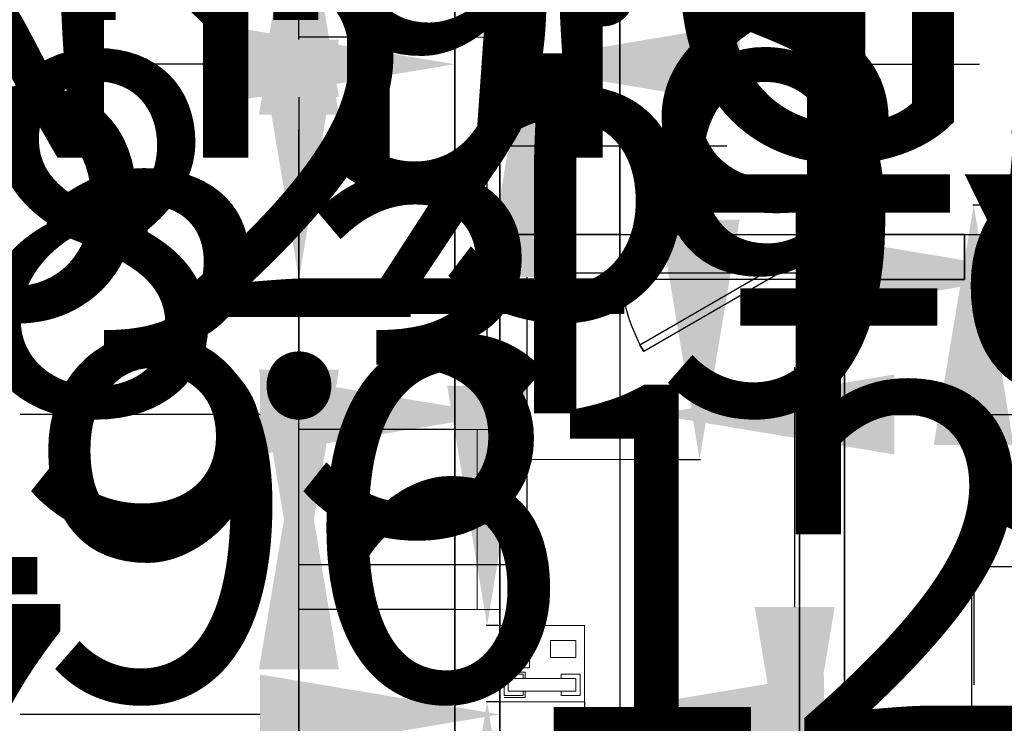
# Model space of a CAD drawing. Units: inches. Extents: x -307 to 2141, y -58 to 895.
# Tile 9 of 28: x 469 to 666, y 312 to 452. Entities that reach past the tile are written whole.
import ezdxf

# ---------------------------------------------------------------- set-up
doc = ezdxf.new("R2010")
doc.units = ezdxf.units.IN
doc.header["$MEASUREMENT"] = 0
for name, color, linetype, lineweight in [('A-ANNO-DIMS', 2, 'Continuous', 18), ('A-DOOR', 3, 'Continuous', 25), ('A-EQPM', 9, 'Continuous', 13), ('A-FLOR-CASE', 32, 'Continuous', 25), ('A-FURN', 8, 'Continuous', 18), ('A-GLAZ', 4, 'Continuous', 18), ('A-WALL', 7, 'Continuous', 35)]:
    doc.layers.add(name, color=color, linetype=linetype, lineweight=lineweight)
doc.styles.get("Standard").update_dxf_attribs({"font": 'arial.ttf'})
doc.dimstyles.get("Standard").update_dxf_attribs({"dimtxt": 72, "dimasz": 48, "dimexe": 0.18, "dimexo": 0.0625, "dimgap": 0.09, "dimtad": 0, "dimtih": 1, "dimtoh": 1, "dimdec": 0, "dimrnd": 48, "dimzin": 0, "dimdsep": 46, "dimlunit": 3, "dimtxsty": 'Standard', "dimcen": 0.09, "dimadec": 0, "dimazin": 0, "dimtfac": 1, "dimtdec": 0, "dimtofl": 0, "dimtmove": 0, "dimatfit": 3, "dimfxl": 1, "dimtolj": 1, "dimtzin": 0, "dimarcsym": 0})

# ---------------------------------------------------------------- blocks, each defined once
blk = doc.blocks.new('*U6')
for p, q in [((0, 0), (0, -6)), ((40, 0), (40, -6))]:
    blk.add_line(p, q)
blk.add_lwpolyline([(0, 0), (34.64, 20), (35.52, 18.48), (0.88, -1.52)], close=True)
blk.add_arc((0, 0), 40, 0, 30)
blk = doc.blocks.new('Phone - Desk')
for p, q in [((-4.5, -5), (-4.5, 5)), ((-4.5, 5), (4.5, 5)), ((4.5, 5), (4.5, -5)), ((-4, 4.5), (-4, 2)), ((-3.75, 4.5), (-3.75, 2.25)), ((-1.25, 4.5), (-3.75, 4.5)), ((-3.25, 4), (-3.25, -4)), ((-3.25, 4), (-1.75, 4)), ((-1.75, -4), (-1.75, 4)), ((-1.25, 2.25), (-1.25, 4.5)), ((-1, 2), (-1, 4.5)), ((4, 3.5), (-0.5, 3.5)), ((-0.5, 3.5), (-0.5, 1.5)), ((4, 1.5), (4, 3.5)), ((-0.5, 2.5), (4, 2.5)), ((-4, 2), (-3.25, 2)), ((-3.75, 2.25), (-3.25, 2.25)), ((-1.75, 2.25), (-1.25, 2.25)), ((-1.75, 2), (-1, 2)), ((-0.5, 1.5), (4, 1.5)), ((2.75, -1), (0.75, -1)), ((0.75, -1), (0.75, -4)), ((2.75, -4), (2.75, -1)), ((-3.75, -2.25), (-3.25, -2.25)), ((-3.75, -4.5), (-3.75, -2.25)), ((-1.75, -2.25), (-1.25, -2.25)), ((-1.25, -2.25), (-1.25, -4.5)), ((-1.25, -4.5), (-3.75, -4.5)), ((-3.25, -4), (-1.75, -4)), ((0.75, -4), (2.75, -4)), ((4.5, -5), (-4.5, -5))]:
    blk.add_line(p, q)
blk = doc.blocks.new('Desk - 30 x 60 in.')
for p, q in [((-26.999995, 0), (26.999995, 0)), ((-29.999995, -27), (-29.999995, -3)), ((29.999995, -3), (29.999995, -27)), ((26.999995, -30), (-26.999995, -30)), ((-20.000005, -30), (-20.000005, -31)), ((-20.000005, -31), (-16.000005, -31)), ((-16.000005, -31), (-16.000005, -30)), ((15.999995, -31), (15.999995, -30)), ((19.999995, -31), (15.999995, -31)), ((19.999995, -30), (19.999995, -31))]:
    blk.add_line(p, q)
for centre, start, end in [((-26.499995, -3.5), 98.1301, 171.8699), ((26.499995, -3.5), 8.130102, 81.8699), ((-26.499995, -26.5), 188.1301, 261.8699), ((26.499995, -26.5), 278.1301, 351.8699)]:
    blk.add_arc(centre, 3.535534, start, end)
blk = doc.blocks.new('WIN-36IN')
for p, q in [((0, 36), (9, 36)), ((4.5, 0), (4.5, 36))]:
    blk.add_line(p, q)
blk.add_lwpolyline([(9, 36), (9, 0), (0, 0), (0, 36)])
blk = doc.blocks.new('*D26')
at = {"layer": 'A-ANNO-DIMS', "color": 0, "lineweight": -2, "transparency": 16777216}
for p, q in [((565.34, 584.2), (565.34, 572.08)), ((645.34, 584.2), (645.34, 572.08)), ((517.34, 572.26), (469.34, 572.26)), ((693.34, 572.26), (741.34, 572.26))]:
    blk.add_line(p, q, dxfattribs=at)
at = {"layer": 'A-ANNO-DIMS', "color": 0, "transparency": 16777216}
for points in [[(517.34, 580.26), (517.34, 564.26), (565.34, 572.26)], [(693.34, 580.26), (693.34, 564.26), (645.34, 572.26)]]:
    blk.add_solid(points, dxfattribs=at)
at = {"layer": 'Defpoints', "color": 0, "transparency": 16777216}
for p in [(565.34, 584.26), (645.34, 584.26), (565.34, 572.26)]:
    blk.add_point(p, dxfattribs=at)
at = {"layer": 'A-ANNO-DIMS', "color": 0, "transparency": 16777216, "insert": (178.23, 572.26), "char_height": 72, "attachment_point": 5}
blk.add_mtext('\\A1;BED 80 TYP.', dxfattribs=at)
blk = doc.blocks.new('*D27')
at = {"layer": 'A-ANNO-DIMS', "color": 0, "lineweight": -2, "transparency": 16777216}
for p, q in [((657.34, 692.26), (657.34, 740.26)), ((645.4, 644.26), (657.52, 644.26)), ((645.4, 584.26), (657.52, 584.26)), ((657.34, 536.26), (657.34, 488.26)), ((657.34, 488.26), (609.34, 488.26))]:
    blk.add_line(p, q, dxfattribs=at)
at = {"layer": 'A-ANNO-DIMS', "color": 0, "transparency": 16777216}
for points in [[(649.34, 692.26), (665.34, 692.26), (657.34, 644.26)], [(649.34, 536.26), (665.34, 536.26), (657.34, 584.26)]]:
    blk.add_solid(points, dxfattribs=at)
at = {"layer": 'Defpoints', "color": 0, "transparency": 16777216}
for p in [(645.34, 644.26), (645.34, 584.26), (657.34, 584.26)]:
    blk.add_point(p, dxfattribs=at)
at = {"layer": 'A-ANNO-DIMS', "color": 0, "transparency": 16777216, "insert": (433.81, 488.26), "char_height": 72, "attachment_point": 5}
blk.add_mtext('\\A1;60 TYP.', dxfattribs=at)
blk = doc.blocks.new('*D28')
at = {"layer": 'A-ANNO-DIMS', "color": 0, "lineweight": -2, "transparency": 16777216}
for p, q in [((795.36, 433.55), (777.92, 433.55)), ((778.1, 385.55), (778.1, 366.07)), ((795.36, 318.07), (777.92, 318.07)), ((778.1, 318.07), (778.1, 270.07)), ((778.1, 270.07), (730.1, 270.07))]:
    blk.add_line(p, q, dxfattribs=at)
at = {"layer": 'A-ANNO-DIMS', "color": 0, "transparency": 16777216}
for points in [[(770.1, 385.55), (786.1, 385.55), (778.1, 433.55)], [(770.1, 366.07), (786.1, 366.07), (778.1, 318.07)]]:
    blk.add_solid(points, dxfattribs=at)
at = {"layer": 'Defpoints', "color": 0, "transparency": 16777216}
for p in [(795.42, 433.55), (778.1, 318.07), (795.42, 318.07)]:
    blk.add_point(p, dxfattribs=at)
at = {"layer": 'A-ANNO-DIMS', "color": 0, "transparency": 16777216, "insert": (534.42, 270.07), "char_height": 72, "attachment_point": 5}
blk.add_mtext('\\A1;BED 115', dxfattribs=at)
blk = doc.blocks.new('*D29')
at = {"layer": 'A-ANNO-DIMS', "color": 0, "lineweight": -2, "transparency": 16777216}
for p, q in [((747.42, 450.87), (699.42, 450.87)), ((795.42, 433.61), (795.42, 451.05)), ((882.03, 433.61), (882.03, 451.05)), ((930.03, 450.87), (978.03, 450.87))]:
    blk.add_line(p, q, dxfattribs=at)
at = {"layer": 'A-ANNO-DIMS', "color": 0, "transparency": 16777216}
for points in [[(747.42, 458.87), (747.42, 442.87), (795.42, 450.87)], [(930.03, 458.87), (930.03, 442.87), (882.03, 450.87)]]:
    blk.add_solid(points, dxfattribs=at)
at = {"layer": 'Defpoints', "color": 0, "transparency": 16777216}
for p in [(795.42, 450.87), (795.42, 433.55), (882.03, 433.55)]:
    blk.add_point(p, dxfattribs=at)
at = {"layer": 'A-ANNO-DIMS', "color": 0, "transparency": 16777216, "insert": (647.71, 450.87), "char_height": 72, "attachment_point": 5}
blk.add_mtext('\\A1;87', dxfattribs=at)
blk = doc.blocks.new('*D30')
at = {"layer": 'A-ANNO-DIMS', "color": 0, "lineweight": -2, "transparency": 16777216}
for p, q in [((570.74, 532.83), (570.74, 580.83)), ((570.74, 580.83), (618.74, 580.83)), ((565.4, 484.83), (570.92, 484.83)), ((565.4, 448.83), (570.92, 448.83)), ((570.74, 400.83), (570.74, 352.83))]:
    blk.add_line(p, q, dxfattribs=at)
at = {"layer": 'A-ANNO-DIMS', "color": 0, "transparency": 16777216}
for points in [[(562.74, 532.83), (578.74, 532.83), (570.74, 484.83)], [(562.74, 400.83), (578.74, 400.83), (570.74, 448.83)]]:
    blk.add_solid(points, dxfattribs=at)
at = {"layer": 'Defpoints', "color": 0, "transparency": 16777216}
for p in [(565.34, 484.83), (570.74, 484.83), (565.34, 448.83)]:
    blk.add_point(p, dxfattribs=at)
at = {"layer": 'A-ANNO-DIMS', "color": 0, "transparency": 16777216, "insert": (1030.17, 580.83), "char_height": 72, "attachment_point": 5}
blk.add_mtext('\\A1;WINDOW 36 TYP.', dxfattribs=at)
blk = doc.blocks.new('*D31')
at = {"layer": 'A-ANNO-DIMS', "color": 0, "lineweight": -2, "transparency": 16777216}
for p, q in [((556.34, 448.77), (556.34, 443.25)), ((565.34, 448.77), (565.34, 443.25)), ((508.34, 443.43), (460.34, 443.43)), ((613.34, 443.43), (661.34, 443.43))]:
    blk.add_line(p, q, dxfattribs=at)
at = {"layer": 'A-ANNO-DIMS', "color": 0, "transparency": 16777216}
for points in [[(508.34, 451.43), (508.34, 435.43), (556.34, 443.43)], [(613.34, 451.43), (613.34, 435.43), (565.34, 443.43)]]:
    blk.add_solid(points, dxfattribs=at)
at = {"layer": 'Defpoints', "color": 0, "transparency": 16777216}
for p in [(556.34, 448.83), (565.34, 448.83), (565.34, 443.43)]:
    blk.add_point(p, dxfattribs=at)
at = {"layer": 'A-ANNO-DIMS', "color": 0, "transparency": 16777216, "insert": (808.69, 443.43), "char_height": 72, "attachment_point": 5}
blk.add_mtext('\\A1;9 TYP.', dxfattribs=at)
blk = doc.blocks.new('*D35')
at = {"layer": 'A-ANNO-DIMS', "color": 0, "lineweight": -2, "transparency": 16777216}
for p, q in [((859.34, 453.77), (811.34, 453.77)), ((907.34, 443.03), (907.34, 453.95)), ((916.34, 443.03), (916.34, 453.95)), ((964.34, 453.77), (1012.34, 453.77))]:
    blk.add_line(p, q, dxfattribs=at)
at = {"layer": 'A-ANNO-DIMS', "color": 0, "transparency": 16777216}
for points in [[(859.34, 461.77), (859.34, 445.77), (907.34, 453.77)], [(964.34, 461.77), (964.34, 445.77), (916.34, 453.77)]]:
    blk.add_solid(points, dxfattribs=at)
at = {"layer": 'Defpoints', "color": 0, "transparency": 16777216}
for p in [(907.34, 453.77), (907.34, 442.97), (916.34, 442.97)]:
    blk.add_point(p, dxfattribs=at)
at = {"layer": 'A-ANNO-DIMS', "color": 0, "transparency": 16777216, "insert": (663.98, 453.77), "char_height": 72, "attachment_point": 5}
blk.add_mtext('\\A1;9 TYP.', dxfattribs=at)
blk = doc.blocks.new('*D36')
at = {"layer": 'A-ANNO-DIMS', "color": 0, "lineweight": -2, "transparency": 16777216}
for p, q in [((871.71, 562.4), (871.76, 610.4)), ((876.55, 514.4), (871.47, 514.4)), ((876.51, 481.35), (871.44, 481.36)), ((871.56, 433.36), (871.51, 385.36)), ((871.51, 385.36), (823.51, 385.36))]:
    blk.add_line(p, q, dxfattribs=at)
at = {"layer": 'A-ANNO-DIMS', "color": 0, "transparency": 16777216}
for points in [[(863.71, 562.41), (879.71, 562.4), (871.65, 514.4)], [(863.56, 433.37), (879.56, 433.35), (871.62, 481.36)]]:
    blk.add_solid(points, dxfattribs=at)
at = {"layer": 'Defpoints', "color": 0, "transparency": 16777216}
for p in [(876.61, 514.4), (871.62, 481.36), (876.57, 481.35)]:
    blk.add_point(p, dxfattribs=at)
at = {"layer": 'A-ANNO-DIMS', "color": 0, "transparency": 16777216, "insert": (548.95, 385.36), "char_height": 72, "attachment_point": 5}
blk.add_mtext('\\A1;WC 33 TYP.', dxfattribs=at)
blk = doc.blocks.new('*D37')
at = {"layer": 'A-ANNO-DIMS', "color": 0, "lineweight": -2, "transparency": 16777216}
for p, q in [((828.62, 519.41), (780.62, 519.46)), ((876.61, 514.46), (876.62, 519.54)), ((897.61, 514.44), (897.62, 519.51)), ((945.62, 519.28), (993.62, 519.22))]:
    blk.add_line(p, q, dxfattribs=at)
at = {"layer": 'A-ANNO-DIMS', "color": 0, "transparency": 16777216}
for points in [[(828.63, 527.41), (828.61, 511.41), (876.62, 519.36)], [(945.63, 527.28), (945.61, 511.28), (897.62, 519.33)]]:
    blk.add_solid(points, dxfattribs=at)
at = {"layer": 'Defpoints', "color": 0, "transparency": 16777216}
for p in [(876.62, 519.36), (876.61, 514.4), (897.61, 514.38)]:
    blk.add_point(p, dxfattribs=at)
at = {"layer": 'A-ANNO-DIMS', "color": 0, "transparency": 16777216, "insert": (604.68, 519.46), "char_height": 72, "attachment_point": 5}
blk.add_mtext('\\A1;21 TYP.', dxfattribs=at)
blk = doc.blocks.new('*D38')
at = {"layer": 'A-ANNO-DIMS', "color": 0, "lineweight": -2, "transparency": 16777216}
for p, q in [((598.5, 222.79), (550.5, 222.79)), ((646.5, 213.85), (646.5, 222.97)), ((706.5, 213.85), (706.5, 222.97)), ((754.5, 222.79), (802.5, 222.79))]:
    blk.add_line(p, q, dxfattribs=at)
at = {"layer": 'A-ANNO-DIMS', "color": 0, "transparency": 16777216}
for points in [[(598.5, 230.79), (598.5, 214.79), (646.5, 222.79)], [(754.5, 230.79), (754.5, 214.79), (706.5, 222.79)]]:
    blk.add_solid(points, dxfattribs=at)
at = {"layer": 'Defpoints', "color": 0, "transparency": 16777216}
for p in [(646.5, 222.79), (646.5, 213.79), (706.5, 213.79)]:
    blk.add_point(p, dxfattribs=at)
at = {"layer": 'A-ANNO-DIMS', "color": 0, "transparency": 16777216, "insert": (97.26, 222.79), "char_height": 72, "attachment_point": 5}
blk.add_mtext('\\A1;LOVESEAT 60 TYP.', dxfattribs=at)
blk = doc.blocks.new('*D48')
at = {"layer": 'A-ANNO-DIMS', "color": 0, "lineweight": -2, "transparency": 16777216}
for p, q in [((724, 313.98), (724, 361.98)), ((732.94, 265.98), (723.82, 265.98)), ((732.94, 205.98), (723.82, 205.98)), ((724, 157.98), (724, 109.98)), ((724, 109.98), (676, 109.98))]:
    blk.add_line(p, q, dxfattribs=at)
at = {"layer": 'A-ANNO-DIMS', "color": 0, "transparency": 16777216}
for points in [[(716, 313.98), (732, 313.98), (724, 265.98)], [(716, 157.98), (732, 157.98), (724, 205.98)]]:
    blk.add_solid(points, dxfattribs=at)
at = {"layer": 'Defpoints', "color": 0, "transparency": 16777216}
for p in [(733, 265.98), (724, 205.98), (733, 205.98)]:
    blk.add_point(p, dxfattribs=at)
at = {"layer": 'A-ANNO-DIMS', "color": 0, "transparency": 16777216, "insert": (321.56, 109.98), "char_height": 72, "attachment_point": 5}
blk.add_mtext('\\A1;MEDIA UNIT 60', dxfattribs=at)
blk = doc.blocks.new('*D50')
at = {"layer": 'A-ANNO-DIMS', "color": 0, "lineweight": -2, "transparency": 16777216}
for p, q in [((565.34, 315.8), (565.34, 313.15)), ((582.27, 315.8), (582.27, 313.15)), ((517.34, 313.33), (469.34, 313.33)), ((630.27, 313.33), (678.27, 313.33))]:
    blk.add_line(p, q, dxfattribs=at)
at = {"layer": 'A-ANNO-DIMS', "color": 0, "transparency": 16777216}
for points in [[(517.34, 321.33), (517.34, 305.33), (565.34, 313.33)], [(630.27, 321.33), (630.27, 305.33), (582.27, 313.33)]]:
    blk.add_solid(points, dxfattribs=at)
at = {"layer": 'Defpoints', "color": 0, "transparency": 16777216}
for p in [(565.34, 315.87), (582.27, 315.87), (565.34, 313.33)]:
    blk.add_point(p, dxfattribs=at)
at = {"layer": 'A-ANNO-DIMS', "color": 0, "transparency": 16777216, "insert": (226.65, 313.33), "char_height": 72, "attachment_point": 5}
blk.add_mtext('\\A1;PHONE 17', dxfattribs=at)
blk = doc.blocks.new('*D51')
at = {"layer": 'A-ANNO-DIMS', "color": 0, "lineweight": -2, "transparency": 16777216}
for p, q in [((562.8, 379.11), (562.8, 427.11)), ((562.8, 427.11), (610.8, 427.11)), ((565.27, 331.11), (562.62, 331.11)), ((565.27, 315.87), (562.62, 315.87)), ((562.8, 267.87), (562.8, 219.87))]:
    blk.add_line(p, q, dxfattribs=at)
at = {"layer": 'A-ANNO-DIMS', "color": 0, "transparency": 16777216}
for points in [[(554.8, 379.11), (570.8, 379.11), (562.8, 331.11)], [(554.8, 267.87), (570.8, 267.87), (562.8, 315.87)]]:
    blk.add_solid(points, dxfattribs=at)
at = {"layer": 'Defpoints', "color": 0, "transparency": 16777216}
for p in [(562.8, 331.11), (565.34, 331.11), (565.34, 315.87)]:
    blk.add_point(p, dxfattribs=at)
at = {"layer": 'A-ANNO-DIMS', "color": 0, "transparency": 16777216, "insert": (659.34, 427.11), "char_height": 72, "attachment_point": 5}
blk.add_mtext('\\A1;15', dxfattribs=at)
blk = doc.blocks.new('*D52')
at = {"layer": 'A-ANNO-DIMS', "color": 0, "lineweight": -2, "transparency": 16777216}
for p, q in [((660.21, 554.25), (660.21, 602.25)), ((673.8, 506.25), (660.03, 506.25)), ((673.8, 415.25), (660.03, 415.25)), ((660.21, 367.25), (660.21, 319.25))]:
    blk.add_line(p, q, dxfattribs=at)
at = {"layer": 'A-ANNO-DIMS', "color": 0, "transparency": 16777216}
for points in [[(652.21, 554.25), (668.21, 554.25), (660.21, 506.25)], [(652.21, 367.25), (668.21, 367.25), (660.21, 415.25)]]:
    blk.add_solid(points, dxfattribs=at)
at = {"layer": 'Defpoints', "color": 0, "transparency": 16777216}
for p in [(673.86, 506.25), (660.21, 415.25), (673.86, 415.25)]:
    blk.add_point(p, dxfattribs=at)
at = {"layer": 'A-ANNO-DIMS', "color": 0, "transparency": 16777216, "insert": (660.21, 460.75), "char_height": 72, "attachment_point": 5}
blk.add_mtext('\\A1;DINING SET 91', dxfattribs=at)
blk = doc.blocks.new('*D53')
at = {"layer": 'A-ANNO-DIMS', "color": 0, "lineweight": -2, "transparency": 16777216}
for p, q in [((673.86, 415.19), (673.86, 401.42)), ((728.86, 415.19), (728.86, 401.42)), ((625.86, 401.6), (577.86, 401.6)), ((776.86, 401.6), (824.86, 401.6))]:
    blk.add_line(p, q, dxfattribs=at)
at = {"layer": 'A-ANNO-DIMS', "color": 0, "transparency": 16777216}
for points in [[(625.86, 409.6), (625.86, 393.6), (673.86, 401.6)], [(776.86, 409.6), (776.86, 393.6), (728.86, 401.6)]]:
    blk.add_solid(points, dxfattribs=at)
at = {"layer": 'Defpoints', "color": 0, "transparency": 16777216}
for p in [(673.86, 415.25), (728.86, 415.25), (728.86, 401.6)]:
    blk.add_point(p, dxfattribs=at)
at = {"layer": 'A-ANNO-DIMS', "color": 0, "transparency": 16777216, "insert": (876.79, 401.6), "char_height": 72, "attachment_point": 5}
blk.add_mtext('\\A1;55', dxfattribs=at)
blk = doc.blocks.new('*D54')
at = {"layer": 'A-ANNO-DIMS', "color": 0, "lineweight": -2, "transparency": 16777216}
for p, q in [((605.34, 412.35), (605.34, 460.35)), ((605.34, 460.35), (653.34, 460.35)), ((596.4, 364.35), (605.52, 364.35)), ((596.4, 304.35), (605.52, 304.35)), ((605.34, 256.35), (605.34, 208.35))]:
    blk.add_line(p, q, dxfattribs=at)
at = {"layer": 'A-ANNO-DIMS', "color": 0, "transparency": 16777216}
for points in [[(597.34, 412.35), (613.34, 412.35), (605.34, 364.35)], [(597.34, 256.35), (613.34, 256.35), (605.34, 304.35)]]:
    blk.add_solid(points, dxfattribs=at)
at = {"layer": 'Defpoints', "color": 0, "transparency": 16777216}
for p in [(596.34, 364.35), (605.34, 364.35), (596.34, 304.35)]:
    blk.add_point(p, dxfattribs=at)
at = {"layer": 'A-ANNO-DIMS', "color": 0, "transparency": 16777216, "insert": (854, 460.35), "char_height": 72, "attachment_point": 5}
blk.add_mtext('\\A1;DESK 60', dxfattribs=at)
blk = doc.blocks.new('*D55')
at = {"layer": 'A-ANNO-DIMS', "color": 0, "lineweight": -2, "transparency": 16777216}
for p, q in [((517.34, 373.35), (469.34, 373.35)), ((565.34, 364.41), (565.34, 373.53)), ((596.34, 364.41), (596.34, 373.53)), ((644.34, 373.35), (692.34, 373.35))]:
    blk.add_line(p, q, dxfattribs=at)
at = {"layer": 'A-ANNO-DIMS', "color": 0, "transparency": 16777216}
for points in [[(517.34, 381.35), (517.34, 365.35), (565.34, 373.35)], [(644.34, 381.35), (644.34, 365.35), (596.34, 373.35)]]:
    blk.add_solid(points, dxfattribs=at)
at = {"layer": 'Defpoints', "color": 0, "transparency": 16777216}
for p in [(565.34, 373.35), (565.34, 364.35), (596.34, 364.35)]:
    blk.add_point(p, dxfattribs=at)
at = {"layer": 'A-ANNO-DIMS', "color": 0, "transparency": 16777216, "insert": (424.65, 373.35), "char_height": 72, "attachment_point": 5}
blk.add_mtext('\\A1;31', dxfattribs=at)
blk = doc.blocks.new('*D58')
at = {"layer": 'A-ANNO-DIMS', "color": 0, "lineweight": -2, "transparency": 16777216}
for p, q in [((624.38, 334.8), (624.38, 382.8)), ((611.84, 286.8), (624.56, 286.8)), ((611.84, 202.8), (624.56, 202.8)), ((624.38, 154.8), (624.38, 106.8))]:
    blk.add_line(p, q, dxfattribs=at)
at = {"layer": 'A-ANNO-DIMS', "color": 0, "transparency": 16777216}
for points in [[(616.38, 334.8), (632.38, 334.8), (624.38, 286.8)], [(616.38, 154.8), (632.38, 154.8), (624.38, 202.8)]]:
    blk.add_solid(points, dxfattribs=at)
at = {"layer": 'Defpoints', "color": 0, "transparency": 16777216}
for p in [(611.78, 286.8), (624.38, 286.8), (611.78, 202.8)]:
    blk.add_point(p, dxfattribs=at)
at = {"layer": 'A-ANNO-DIMS', "color": 0, "transparency": 16777216, "insert": (624.38, 244.8), "char_height": 72, "attachment_point": 5}
blk.add_mtext('\\A1;SOFA 84', dxfattribs=at)
blk = doc.blocks.new('*D59')
at = {"layer": 'A-ANNO-DIMS', "color": 0, "lineweight": -2, "transparency": 16777216}
for p, q in [((527.11, 299.4), (479.11, 299.4)), ((575.11, 286.86), (575.11, 299.58)), ((611.78, 286.86), (611.78, 299.58)), ((659.78, 299.4), (707.78, 299.4))]:
    blk.add_line(p, q, dxfattribs=at)
at = {"layer": 'A-ANNO-DIMS', "color": 0, "transparency": 16777216}
for points in [[(527.11, 307.4), (527.11, 291.4), (575.11, 299.4)], [(659.78, 307.4), (659.78, 291.4), (611.78, 299.4)]]:
    blk.add_solid(points, dxfattribs=at)
at = {"layer": 'Defpoints', "color": 0, "transparency": 16777216}
for p in [(575.11, 299.4), (575.11, 286.8), (611.78, 286.8)]:
    blk.add_point(p, dxfattribs=at)
at = {"layer": 'A-ANNO-DIMS', "color": 0, "transparency": 16777216, "insert": (427.48, 299.4), "char_height": 72, "attachment_point": 5}
blk.add_mtext('\\A1;37', dxfattribs=at)
blk = doc.blocks.new('*D60')
at = {"layer": 'A-ANNO-DIMS', "color": 0, "lineweight": -2, "transparency": 16777216}
for p, q in [((659.86, 294.95), (659.86, 342.95)), ((659.86, 342.95), (707.86, 342.95)), ((663.34, 246.95), (659.68, 246.95)), ((663.34, 223.32), (659.68, 223.32)), ((659.86, 175.32), (659.86, 127.32))]:
    blk.add_line(p, q, dxfattribs=at)
at = {"layer": 'A-ANNO-DIMS', "color": 0, "transparency": 16777216}
for points in [[(651.86, 294.95), (667.86, 294.95), (659.86, 246.95)], [(651.86, 175.32), (667.86, 175.32), (659.86, 223.32)]]:
    blk.add_solid(points, dxfattribs=at)
at = {"layer": 'Defpoints', "color": 0, "transparency": 16777216}
for p in [(659.86, 246.95), (663.4, 246.95), (663.4, 223.32)]:
    blk.add_point(p, dxfattribs=at)
at = {"layer": 'A-ANNO-DIMS', "color": 0, "transparency": 16777216, "insert": (933.57, 342.95), "char_height": 72, "attachment_point": 5}
blk.add_mtext('\\A1;TABLE 24', dxfattribs=at)
blk = doc.blocks.new('*D64')
at = {"layer": 'A-ANNO-DIMS', "color": 0, "lineweight": -2, "transparency": 16777216}
for p, q in [((556.27, 691.34), (524.95, 691.34)), ((525.13, 643.34), (525.13, 465.69)), ((525.13, 214.34), (525.13, 391.99)), ((556.27, 166.34), (524.95, 166.34))]:
    blk.add_line(p, q, dxfattribs=at)
at = {"layer": 'A-ANNO-DIMS', "color": 0, "transparency": 16777216}
for points in [[(517.13, 643.34), (533.13, 643.34), (525.13, 691.34)], [(517.13, 214.34), (533.13, 214.34), (525.13, 166.34)]]:
    blk.add_solid(points, dxfattribs=at)
at = {"layer": 'Defpoints', "color": 0, "transparency": 16777216}
for p in [(525.13, 691.34), (556.34, 691.34), (556.34, 166.34)]:
    blk.add_point(p, dxfattribs=at)
at = {"layer": 'A-ANNO-DIMS', "color": 0, "transparency": 16777216, "insert": (525.13, 428.84), "char_height": 72, "attachment_point": 5}
blk.add_mtext('\\A1;525', dxfattribs=at)
blk = doc.blocks.new('*D66')
at = {"layer": 'A-ANNO-DIMS', "color": 0, "lineweight": -2, "transparency": 16777216}
for p, q in [((525.13, 382.34), (525.13, 430.34)), ((556.27, 334.34), (524.95, 334.34)), ((565.27, 304.34), (524.95, 304.34)), ((525.13, 256.34), (525.13, 208.34)), ((525.13, 208.34), (477.13, 208.34))]:
    blk.add_line(p, q, dxfattribs=at)
at = {"layer": 'A-ANNO-DIMS', "color": 0, "transparency": 16777216}
for points in [[(517.13, 382.34), (533.13, 382.34), (525.13, 334.34)], [(517.13, 256.34), (533.13, 256.34), (525.13, 304.34)]]:
    blk.add_solid(points, dxfattribs=at)
at = {"layer": 'Defpoints', "color": 0, "transparency": 16777216}
for p in [(556.34, 334.34), (525.13, 304.34), (565.34, 304.34)]:
    blk.add_point(p, dxfattribs=at)
at = {"layer": 'A-ANNO-DIMS', "color": 0, "transparency": 16777216, "insert": (425.62, 208.34), "char_height": 72, "attachment_point": 5}
blk.add_mtext('\\A1;30', dxfattribs=at)
blk = doc.blocks.new('*D67')
at = {"layer": 'A-ANNO-DIMS', "color": 0, "lineweight": -2, "transparency": 16777216}
for p, q in [((525.13, 496.83), (525.13, 544.83)), ((556.27, 448.83), (524.95, 448.83)), ((556.27, 370.34), (524.95, 370.34)), ((525.13, 322.34), (525.13, 274.34))]:
    blk.add_line(p, q, dxfattribs=at)
at = {"layer": 'A-ANNO-DIMS', "color": 0, "transparency": 16777216}
for points in [[(517.13, 496.83), (533.13, 496.83), (525.13, 448.83)], [(517.13, 322.34), (533.13, 322.34), (525.13, 370.34)]]:
    blk.add_solid(points, dxfattribs=at)
at = {"layer": 'Defpoints', "color": 0, "transparency": 16777216}
for p in [(525.13, 448.83), (556.34, 448.83), (556.34, 370.34)]:
    blk.add_point(p, dxfattribs=at)
at = {"layer": 'A-ANNO-DIMS', "color": 0, "transparency": 16777216, "insert": (525.13, 409.59), "char_height": 72, "attachment_point": 5}
blk.add_mtext('\\A1;78.49', dxfattribs=at)
blk = doc.blocks.new('*D68')
at = {"layer": 'A-ANNO-DIMS', "color": 0, "lineweight": -2, "transparency": 16777216}
for p, q in [((525.13, 586.34), (525.13, 634.34)), ((525.13, 634.34), (573.13, 634.34)), ((565.27, 538.34), (524.95, 538.34)), ((556.27, 484.83), (524.95, 484.83)), ((525.13, 436.83), (525.13, 388.83))]:
    blk.add_line(p, q, dxfattribs=at)
at = {"layer": 'A-ANNO-DIMS', "color": 0, "transparency": 16777216}
for points in [[(517.13, 586.34), (533.13, 586.34), (525.13, 538.34)], [(517.13, 436.83), (533.13, 436.83), (525.13, 484.83)]]:
    blk.add_solid(points, dxfattribs=at)
at = {"layer": 'Defpoints', "color": 0, "transparency": 16777216}
for p in [(525.13, 538.34), (565.34, 538.34), (556.34, 484.83)]:
    blk.add_point(p, dxfattribs=at)
at = {"layer": 'A-ANNO-DIMS', "color": 0, "transparency": 16777216, "insert": (687.75, 634.34), "char_height": 72, "attachment_point": 5}
blk.add_mtext('\\A1;53.51', dxfattribs=at)
blk = doc.blocks.new('*D82')
at = {"layer": 'A-ANNO-DIMS', "color": 0, "lineweight": -2, "transparency": 16777216}
for p, q in [((525.13, 565.34), (525.13, 613.34)), ((525.13, 613.34), (573.13, 613.34)), ((802.27, 517.34), (524.95, 517.34)), ((802.27, 481.34), (524.95, 481.34)), ((525.13, 433.34), (525.13, 385.34))]:
    blk.add_line(p, q, dxfattribs=at)
at = {"layer": 'A-ANNO-DIMS', "color": 0, "transparency": 16777216}
for points in [[(517.13, 565.34), (533.13, 565.34), (525.13, 517.34)], [(517.13, 433.34), (533.13, 433.34), (525.13, 481.34)]]:
    blk.add_solid(points, dxfattribs=at)
at = {"layer": 'Defpoints', "color": 0, "transparency": 16777216}
for p in [(525.13, 517.34), (802.34, 517.34), (802.34, 481.34)]:
    blk.add_point(p, dxfattribs=at)
at = {"layer": 'A-ANNO-DIMS', "color": 0, "transparency": 16777216, "insert": (624.74, 613.34), "char_height": 72, "attachment_point": 5}
blk.add_mtext('\\A1;36', dxfattribs=at)
blk = doc.blocks.new('*D83')
at = {"layer": 'A-ANNO-DIMS', "color": 0, "lineweight": -2, "transparency": 16777216}
for p, q in [((947.54, 538.9), (947.54, 586.9)), ((916.4, 490.9), (947.72, 490.9)), ((907.4, 481.34), (947.72, 481.34)), ((947.54, 433.34), (947.54, 385.34)), ((947.54, 385.34), (899.54, 385.34))]:
    blk.add_line(p, q, dxfattribs=at)
at = {"layer": 'A-ANNO-DIMS', "color": 0, "transparency": 16777216}
for points in [[(939.54, 538.9), (955.54, 538.9), (947.54, 490.9)], [(939.54, 433.34), (955.54, 433.34), (947.54, 481.34)]]:
    blk.add_solid(points, dxfattribs=at)
at = {"layer": 'Defpoints', "color": 0, "transparency": 16777216}
for p in [(916.34, 490.9), (907.34, 481.34), (947.54, 481.34)]:
    blk.add_point(p, dxfattribs=at)
at = {"layer": 'A-ANNO-DIMS', "color": 0, "transparency": 16777216, "insert": (777.97, 385.34), "char_height": 72, "attachment_point": 5}
blk.add_mtext('\\A1;9.563', dxfattribs=at)
blk = doc.blocks.new('*D87')
at = {"layer": 'A-ANNO-DIMS', "color": 0, "lineweight": -2, "transparency": 16777216}
for p, q in [((525.13184, 448.340828), (525.13184, 496.340828)), ((625.27334, 400.340828), (524.95184, 400.340828)), ((625.27334, 304.340828), (524.95184, 304.340828)), ((525.13184, 256.340828), (525.13184, 208.340828))]:
    blk.add_line(p, q, dxfattribs=at)
at = {"layer": 'A-ANNO-DIMS', "color": 0, "transparency": 16777216}
for points in [[(517.13184, 448.340828), (533.13184, 448.340828), (525.13184, 400.340828)], [(517.13184, 256.340828), (533.13184, 256.340828), (525.13184, 304.340828)]]:
    blk.add_solid(points, dxfattribs=at)
at = {"layer": 'Defpoints', "color": 0, "transparency": 16777216}
for p in [(525.13184, 400.340828), (625.33584, 400.340828), (625.33584, 304.340828)]:
    blk.add_point(p, dxfattribs=at)
at = {"layer": 'A-ANNO-DIMS', "color": 0, "transparency": 16777216, "insert": (525.13184, 352.340828), "char_height": 72, "attachment_point": 5}
blk.add_mtext('\\A1;96', dxfattribs=at)
blk = doc.blocks.new('*D88')
at = {"layer": 'A-ANNO-DIMS', "color": 0, "lineweight": -2, "transparency": 16777216}
for p, q in [((517.33584, 722.544828), (469.33584, 722.544828)), ((565.33584, 295.403328), (565.33584, 722.724828)), ((754.33584, 271.403328), (754.33584, 722.724828)), ((802.33584, 722.544828), (850.33584, 722.544828))]:
    blk.add_line(p, q, dxfattribs=at)
at = {"layer": 'A-ANNO-DIMS', "color": 0, "transparency": 16777216}
for points in [[(517.33584, 730.544828), (517.33584, 714.544828), (565.33584, 722.544828)], [(802.33584, 730.544828), (802.33584, 714.544828), (754.33584, 722.544828)]]:
    blk.add_solid(points, dxfattribs=at)
at = {"layer": 'Defpoints', "color": 0, "transparency": 16777216}
for p in [(754.33584, 722.544828), (565.33584, 295.340828), (754.33584, 271.340828)]:
    blk.add_point(p, dxfattribs=at)
at = {"layer": 'A-ANNO-DIMS', "color": 0, "transparency": 16777216, "insert": (659.83584, 722.544828), "char_height": 72, "attachment_point": 5}
blk.add_mtext('\\A1;189', dxfattribs=at)
blk = doc.blocks.new('*D89')
at = {"layer": 'A-ANNO-DIMS', "color": 0, "lineweight": -2, "transparency": 16777216}
for p, q in [((525.13, 295.34), (525.13, 343.34)), ((525.13, 343.34), (573.13, 343.34)), ((565.27, 295.34), (524.95, 295.34)), ((525.13, 223.34), (525.13, 247.34)), ((556.27, 175.34), (524.95, 175.34))]:
    blk.add_line(p, q, dxfattribs=at)
at = {"layer": 'A-ANNO-DIMS', "color": 0, "transparency": 16777216}
for points in [[(517.13, 247.34), (533.13, 247.34), (525.13, 295.34)], [(517.13, 223.34), (533.13, 223.34), (525.13, 175.34)]]:
    blk.add_solid(points, dxfattribs=at)
at = {"layer": 'Defpoints', "color": 0, "transparency": 16777216}
for p in [(525.13, 295.34), (565.34, 295.34), (556.34, 175.34)]:
    blk.add_point(p, dxfattribs=at)
at = {"layer": 'A-ANNO-DIMS', "color": 0, "transparency": 16777216, "insert": (649.25, 343.34), "char_height": 72, "attachment_point": 5}
blk.add_mtext('\\A1;120', dxfattribs=at)
blk = doc.blocks.new('*D95')
at = {"layer": 'A-ANNO-DIMS', "color": 0, "lineweight": -2, "transparency": 16777216}
for p, q in [((947.54, 577.34), (947.54, 625.34)), ((947.54, 625.34), (995.54, 625.34)), ((629.9, 529.34), (947.72, 529.34)), ((629.9, 502.66), (947.72, 502.66)), ((947.54, 454.66), (947.54, 406.66))]:
    blk.add_line(p, q, dxfattribs=at)
at = {"layer": 'A-ANNO-DIMS', "color": 0, "transparency": 16777216}
for points in [[(939.54, 577.34), (955.54, 577.34), (947.54, 529.34)], [(939.54, 454.66), (955.54, 454.66), (947.54, 502.66)]]:
    blk.add_solid(points, dxfattribs=at)
at = {"layer": 'Defpoints', "color": 0, "transparency": 16777216}
for p in [(629.84, 529.34), (947.54, 529.34), (629.84, 502.66)]:
    blk.add_point(p, dxfattribs=at)
at = {"layer": 'A-ANNO-DIMS', "color": 0, "transparency": 16777216, "insert": (1117.8, 625.34), "char_height": 72, "attachment_point": 5}
blk.add_mtext('\\A1;26.68', dxfattribs=at)
blk = doc.blocks.new('*D100')
at = {"layer": 'A-ANNO-DIMS', "color": 0, "lineweight": -2, "transparency": 16777216}
for p, q in [((589.34, 409.28), (589.34, 35.96)), ((625.34, 409.28), (625.34, 35.96)), ((541.34, 36.14), (493.34, 36.14)), ((673.34, 36.14), (721.34, 36.14))]:
    blk.add_line(p, q, dxfattribs=at)
at = {"layer": 'A-ANNO-DIMS', "color": 0, "transparency": 16777216}
for points in [[(541.34, 44.14), (541.34, 28.14), (589.34, 36.14)], [(673.34, 44.14), (673.34, 28.14), (625.34, 36.14)]]:
    blk.add_solid(points, dxfattribs=at)
at = {"layer": 'Defpoints', "color": 0, "transparency": 16777216}
for p in [(589.34, 409.34), (625.34, 409.34), (625.34, 36.14)]:
    blk.add_point(p, dxfattribs=at)
at = {"layer": 'A-ANNO-DIMS', "color": 0, "transparency": 16777216, "insert": (772.95, 36.14), "char_height": 72, "attachment_point": 5}
blk.add_mtext('\\A1;36', dxfattribs=at)
blk = doc.blocks.new('*D107')
at = {"layer": 'A-ANNO-DIMS', "color": 0, "lineweight": -2, "transparency": 16777216}
for p, q in [((517.34, 722.54), (469.34, 722.54)), ((565.34, 409.4), (565.34, 722.72)), ((589.34, 409.4), (589.34, 722.72)), ((637.34, 722.54), (685.34, 722.54))]:
    blk.add_line(p, q, dxfattribs=at)
at = {"layer": 'A-ANNO-DIMS', "color": 0, "transparency": 16777216}
for points in [[(517.34, 730.54), (517.34, 714.54), (565.34, 722.54)], [(637.34, 730.54), (637.34, 714.54), (589.34, 722.54)]]:
    blk.add_solid(points, dxfattribs=at)
at = {"layer": 'Defpoints', "color": 0, "transparency": 16777216}
for p in [(589.34, 722.54), (565.34, 409.34), (589.34, 409.34)]:
    blk.add_point(p, dxfattribs=at)
at = {"layer": 'A-ANNO-DIMS', "color": 0, "transparency": 16777216, "insert": (835.49, 722.54), "char_height": 72, "attachment_point": 5}
blk.add_mtext('\\A1;24.003', dxfattribs=at)
blk = doc.blocks.new('*D108')
at = {"layer": 'A-ANNO-DIMS', "color": 0, "lineweight": -2, "transparency": 16777216}
for p, q in [((947.54, 550.66), (947.54, 598.66)), ((589.4, 502.66), (947.72, 502.66)), ((589.4, 409.34), (947.72, 409.34)), ((947.54, 361.34), (947.54, 313.34))]:
    blk.add_line(p, q, dxfattribs=at)
at = {"layer": 'A-ANNO-DIMS', "color": 0, "transparency": 16777216}
for points in [[(939.54, 550.66), (955.54, 550.66), (947.54, 502.66)], [(939.54, 361.34), (955.54, 361.34), (947.54, 409.34)]]:
    blk.add_solid(points, dxfattribs=at)
at = {"layer": 'Defpoints', "color": 0, "transparency": 16777216}
for p in [(589.34, 502.66), (947.54, 502.66), (589.34, 409.34)]:
    blk.add_point(p, dxfattribs=at)
at = {"layer": 'A-ANNO-DIMS', "color": 0, "transparency": 16777216, "insert": (947.54, 456), "char_height": 72, "attachment_point": 5}
blk.add_mtext('\\A1;93.32', dxfattribs=at)

msp = doc.modelspace()

# ---------------------------------------------------------------- linework, layer by layer
at = {"layer": 'A-FLOR-CASE'}
msp.add_lwpolyline([(589.339, 502.6632), (589.339, 409.3408), (565.3358, 409.3408), (565.3358, 529.3408), (589.339, 529.3408)], dxfattribs=at)
at = {"layer": 'A-WALL'}
for p, q in [((556.3358, 691.3408), (556.3358, 91.3408)), ((565.3358, 682.3408), (565.3358, 100.3408)), ((589.3358, 409.3408), (565.3358, 409.3408)), ((589.3358, 400.3408), (589.3358, 409.3408)), ((658.3358, 409.3408), (625.3358, 409.3408)), ((625.3358, 400.3408), (625.3358, 409.3408)), ((658.3358, 409.3408), (658.3358, 400.3408)), ((589.3358, 400.3408), (565.3358, 400.3408)), ((625.3358, 400.3408), (625.3358, 304.3408)), ((658.3358, 400.3408), (634.3358, 400.3408)), ((634.3358, 400.3408), (634.3358, 295.3408))]:
    msp.add_line(p, q, dxfattribs=at)

# ---------------------------------------------------------------- block references
at = {"layer": 'A-DOOR', "xscale": 0.899920095740209, "yscale": 0.899920095740209, "zscale": 0.899920095740209, "rotation": 179.9999999999999}
msp.add_blockref('*U6', (625.3358, 403.9413), dxfattribs=at)
at = {"layer": 'A-EQPM', "xscale": 1.693553955443994, "yscale": 1.693553955443994, "zscale": 1.693553955443994, "rotation": 90}
msp.add_blockref('Phone - Desk', (573.8036, 323.4876), dxfattribs=at)
at = {"layer": 'A-FURN', "rotation": 90}
msp.add_blockref('Desk - 30 x 60 in.', (565.3358, 334.3488), dxfattribs=at)
at = {"layer": 'A-GLAZ'}
for p in [(556.336, 448.8337), (556.336, 334.342)]:
    msp.add_blockref('WIN-36IN', p, dxfattribs=at)

# ---------------------------------------------------------------- dimensions: what is measured, and where the dimension line sits
at = {"layer": 'A-ANNO-DIMS'}
for base, p1, p2, override, picture, middle in [((754.3358, 722.5448), (565.3358, 295.3408), (754.3358, 271.3408), {"dimdec": 0, "dimlfac": 1, "dimrnd": 0, "dimzin": 0, "dimdsep": 46, "dimlunit": 2}, '*D88', (659.8358, 722.5448)), ((589.339, 722.5448), (565.3358, 409.3408), (589.339, 409.3408), {"dimdec": 3, "dimlfac": 1, "dimrnd": 0, "dimzin": 0, "dimdsep": 46, "dimlunit": 2}, '*D107', (835.4945, 722.5448)), ((728.8583, 401.5985), (673.8583, 415.2485), (728.8583, 415.2485), {"dimdec": 0, "dimlfac": 1, "dimrnd": 0, "dimzin": 0, "dimdsep": 46, "dimlunit": 2}, '*D53', (876.7874, 401.5985)), ((625.3358, 36.1368), (589.339, 409.3408), (625.3358, 409.3408), {"dimdec": 0, "dimlfac": 1, "dimrnd": 0, "dimzin": 0, "dimdsep": 46, "dimlunit": 2}, '*D100', (772.9456, 36.1368))]:
    dim = msp.add_linear_dim(base=base, p1=p1, p2=p2, dimstyle='Standard', override=override, dxfattribs=at)
    dim.commit()
    dim.dimension.update_dxf_attribs({"geometry": picture, "text_midpoint": middle})
for base, p1, p2, angle, text, picture, middle in [((570.7358, 484.8333), (565.3358, 448.8333), (565.3358, 484.8333), 90, 'WINDOW <> TYP.', '*D30', (1030.1737, 580.8333)), ((565.3358, 572.2648), (645.3359, 584.2648), (565.3358, 584.2648), 180, 'BED <> TYP.', '*D26', (178.2254, 572.2648)), ((657.3359, 584.2648), (645.3359, 644.2648), (645.3359, 584.2648), 270, '<> TYP.', '*D27', (433.8134, 488.2648)), ((660.2083, 415.2485), (673.8583, 506.2485), (673.8583, 415.2485), 270, 'DINING SET <>', '*D52', (660.2083, 460.7485)), ((876.6162, 519.3557), (897.6106, 514.3753), (876.6106, 514.3988), 179.935892, '<> TYP.', '*D37', (604.6763, 519.4631)), ((871.6167, 481.3581), (876.6106, 514.3988), (876.5736, 481.3526), 269.935892, 'WC <> TYP.', '*D36', (548.95, 385.3582)), ((605.3358, 364.3488), (596.3358, 304.3488), (596.3358, 364.3488), 90, 'DESK <>', '*D54', (854.0043, 460.3488)), ((907.3358, 453.7692), (916.3358, 442.9669), (907.3358, 442.9669), 180, '<> TYP.', '*D35', (663.9798, 453.7692)), ((659.8571, 246.9465), (663.4018, 223.3153), (663.4018, 246.9465), 90, 'TABLE <>', '*D60', (933.5733, 342.9465)), ((778.0993, 318.073), (795.4208, 433.5496), (795.4208, 318.073), 270, 'BED <>', '*D28', (534.4158, 270.073)), ((565.3358, 313.3263), (582.2714, 315.8666), (565.3358, 315.8666), 180, 'PHONE <>', '*D50', (226.651, 313.3263)), ((646.4965, 222.7908), (706.4965, 213.7908), (646.4965, 213.7908), 180, 'LOVESEAT <> TYP.', '*D38', (97.2632, 222.7908)), ((624.377, 286.7976), (611.777, 202.7976), (611.777, 286.7976), 90, 'SOFA <>', '*D58', (624.377, 244.7976)), ((724.0025, 205.9815), (733.0025, 265.9815), (733.0025, 205.9815), 270, 'MEDIA UNIT <>', '*D48', (321.5605, 109.9815))]:
    dim = msp.add_linear_dim(base=base, p1=p1, p2=p2, angle=angle, text=text, dimstyle='Standard', override={"dimdec": 0, "dimlfac": 1, "dimrnd": 0, "dimzin": 0, "dimdsep": 46, "dimlunit": 2}, dxfattribs=at)
    dim.commit()
    dim.dimension.update_dxf_attribs({"geometry": picture, "text_midpoint": middle})
for base, p1, p2, angle, override, picture, middle in [((525.1318, 691.3408), (556.3358, 166.3408), (556.3358, 691.3408), 90, {"dimdec": 0, "dimlfac": 1, "dimrnd": 0, "dimzin": 0, "dimdsep": 46, "dimlunit": 2}, '*D64', (525.1318, 428.8408)), ((525.1318, 538.3408), (556.3358, 484.8333), (565.3358, 538.3408), 90, {"dimdec": 2, "dimlfac": 1, "dimrnd": 0, "dimzin": 0, "dimdsep": 46, "dimlunit": 2}, '*D68', (687.7539, 634.3408)), ((947.5398, 529.3408), (629.8358, 502.6632), (629.8358, 529.3408), 90, {"dimdec": 2, "dimlfac": 1, "dimrnd": 0, "dimzin": 0, "dimdsep": 46, "dimlunit": 2}, '*D95', (1117.799, 625.3408)), ((525.1318, 517.3408), (802.3358, 481.3408), (802.3358, 517.3408), 90, {"dimdec": 0, "dimlfac": 1, "dimrnd": 0, "dimzin": 0, "dimdsep": 46, "dimlunit": 2}, '*D82', (624.7416, 613.3408)), ((947.5398, 502.6632), (589.339, 409.3408), (589.339, 502.6632), 90, {"dimdec": 2, "dimlfac": 1, "dimrnd": 0, "dimzin": 0, "dimdsep": 46, "dimlunit": 2}, '*D108', (947.5398, 456.002)), ((947.5398, 481.3408), (916.3358, 490.9034), (907.3358, 481.3408), 90, {"dimdec": 3, "dimlfac": 1, "dimrnd": 0, "dimzin": 0, "dimdsep": 46, "dimlunit": 2}, '*D83', (777.9683, 385.3408)), ((525.1318, 448.8333), (556.3358, 370.3416), (556.3358, 448.8333), 90, {"dimdec": 2, "dimlfac": 1, "dimrnd": 0, "dimzin": 0, "dimdsep": 46, "dimlunit": 2}, '*D67', (525.1318, 409.5874)), ((795.4208, 450.8711), (882.0282, 433.5496), (795.4208, 433.5496), 180, {"dimdec": 0, "dimlfac": 1, "dimrnd": 0, "dimzin": 0, "dimdsep": 46, "dimlunit": 2}, '*D29', (647.7128, 450.8711)), ((525.1318, 400.3408), (625.3358, 304.3408), (625.3358, 400.3408), 90, {"dimdec": 0, "dimlfac": 1, "dimrnd": 0, "dimzin": 0, "dimdsep": 46, "dimlunit": 2}, '*D87', (525.1318, 352.3408)), ((562.7955, 331.1086), (565.3358, 315.8666), (565.3358, 331.1086), 90, {"dimdec": 0, "dimlfac": 1, "dimrnd": 0, "dimzin": 0, "dimdsep": 46, "dimlunit": 2}, '*D51', (659.3357, 427.1086)), ((525.1318, 304.3408), (556.3358, 334.3416), (565.3358, 304.3408), 90, {"dimdec": 0, "dimlfac": 1, "dimrnd": 0, "dimzin": 0, "dimdsep": 46, "dimlunit": 2}, '*D66', (425.6203, 208.3408)), ((565.3358, 373.3488), (596.3358, 364.3488), (565.3358, 364.3488), 180, {"dimdec": 0, "dimlfac": 1, "dimrnd": 0, "dimzin": 0, "dimdsep": 46, "dimlunit": 2}, '*D55', (424.651, 373.3488)), ((525.1318, 295.3408), (556.3358, 175.3408), (565.3358, 295.3408), 90, {"dimdec": 0, "dimlfac": 1, "dimrnd": 0, "dimzin": 0, "dimdsep": 46, "dimlunit": 2}, '*D89', (649.2491, 343.3408)), ((575.1104, 299.3976), (611.777, 286.7976), (575.1104, 286.7976), 180, {"dimdec": 0, "dimlfac": 1, "dimrnd": 0, "dimzin": 0, "dimdsep": 46, "dimlunit": 2}, '*D59', (427.476, 299.3976))]:
    dim = msp.add_linear_dim(base=base, p1=p1, p2=p2, angle=angle, dimstyle='Standard', override=override, dxfattribs=at)
    dim.commit()
    dim.dimension.update_dxf_attribs({"geometry": picture, "text_midpoint": middle})
dim = msp.add_linear_dim(base=(565.3358, 443.4333), p1=(556.3358, 448.8333), p2=(565.3358, 448.8333), text='<> TYP.', dimstyle='Standard', override={"dimdec": 0, "dimlfac": 1, "dimrnd": 0, "dimzin": 0, "dimdsep": 46, "dimlunit": 2}, dxfattribs=at)
dim.commit()
dim.dimension.update_dxf_attribs({"geometry": '*D31', "text_midpoint": (808.6919, 443.4333)})

doc.saveas('drawing.dxf')
